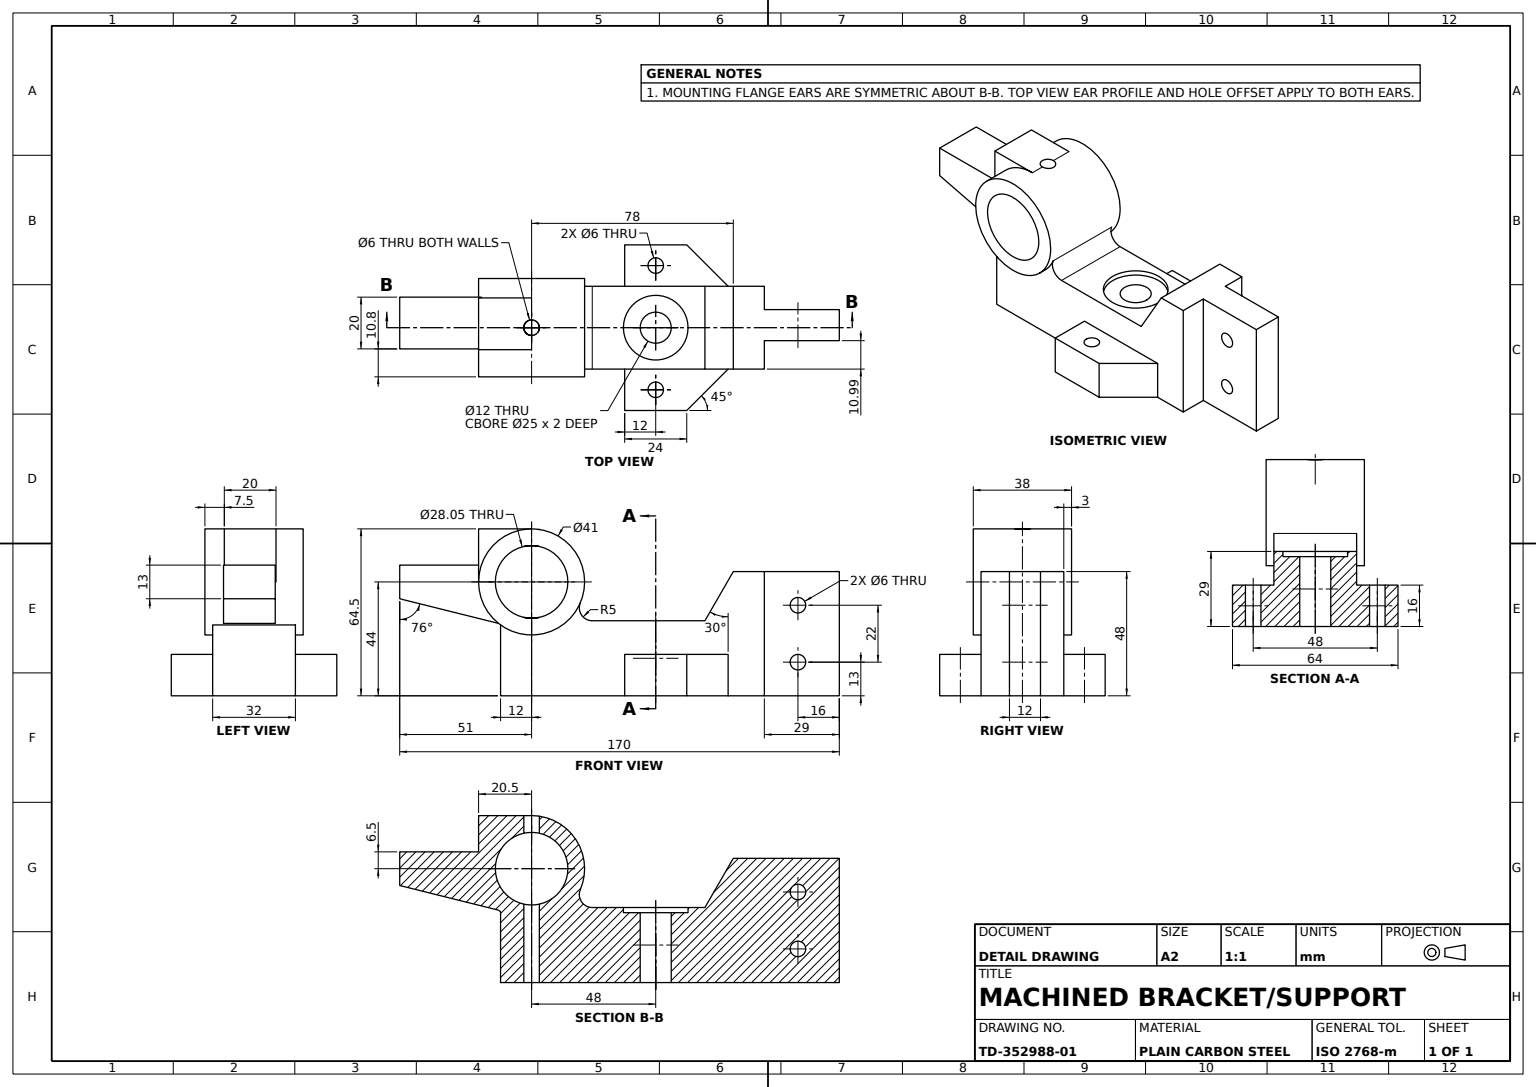
SolidWorks part; units mm, degrees
material "Plain Carbon Steel"
ref_plane "Front Plane" through (0, 0, 0) normal (0, 0, 1) x (1, 0, 0)
ref_plane "Top Plane" through (0, 0, 0) normal (0, 1, 0) x (1, 0, 0)
ref_plane "Right Plane" through (0, 0, 0) normal (1, 0, 0) x (0, 0, -1)
sketch "Base Block Sketch" plane through (0, 0, 0) normal (0, 1, 0) x (1, 0, 0)
  line L0 (-16.6126, 0) -> (35.5105, 0) construction
  line L1 (12, 0) -> (41, 0)
  line L3 (12, 12) -> (41, 12)
  line L4 (41, 0) -> (41, 12)
  line L9 (0, 23.3887) -> (0, -17.813) construction
  line L10 (0, 6) -> (46.308, 6) construction
  line L11 (0, -10.986) -> (12, -10.986)
  line L12 (0, -10.986) -> (0, 21.014)
  line L13 (0, 21.014) -> (12, 21.014)
  line L14 (12, -10.986) -> (12, 0)
  line L15 (12, 12) -> (12, 21.014)
  dimension "D1" = 12
  dimension "D2" = 41
  dimension "D3" = 12
  dimension "D4" = 32
  dimension "D5" = 10.986
  dimension "D6" = 2.3746
  dimension "D7" = 6.827
  dimension "D8" = 16.6126
  dimension "D9" = 5.4895
  dimension "D10" = 6
extrude "Base Block 48mm" add sketch "Base Block Sketch" along normal blind 48
sketch "Base Notch Sketch" plane through (0, 0, 0) normal (0, 0, 1) x (1, 0, 0)
  line L0 (25, 53.5167) -> (25, -6.2579) construction
  line L4 (12, 0) -> (41, 0) construction
  circle A0 centre (25, 35) radius 3
  circle A1 centre (25, 13) radius 3
  dimension "D4" = 6
  dimension "D1" = 25
  dimension "D2" = 22
  dimension "D3" = 13
extrude "Base Notch Cut" cut sketch "Base Notch Sketch" against normal through all
sketch "Angled Arm Sketch" plane through (0, 0, 10.986) normal (0, 0, 1) x (1, 0, 0)
  line L0 (0, 48) -> (-10.9697, 29)
  line L1 (-10.9697, 29) -> (-90, 29)
  line L2 (-90, 29) -> (-90, 0)
  line L3 (-90, 0) -> (0, 0)
  line L4 (12, 48) -> (12, 0) construction
  line L5 (0, 0) -> (0, 48)
  dimension "D1" = 90
  dimension "D2" = 30
  dimension "D3" = 29
extrude "Angled Arm 30deg" add sketch "Angled Arm Sketch" against normal blind 32
sketch "Mounting Flange Sketch" plane through (0, 0, 10.986) normal (0, 0, 1) x (1, 0, 0)
  line L0 (-78, 0) -> (-78, 44) construction
  line L1 (-90, 0) -> (12, 0) construction
  circle A0 centre (-78, 44) radius 20.5
  circle A1 centre (-78, 44) radius 14
  dimension "D3" = 41
  dimension "D4" = 28
  dimension "D1" = 12
  dimension "D2" = 44
extrude "Mounting Flange" add sketch "Mounting Flange Sketch" against normal blind 35 and the other way blind 3
sketch "Raised Block Sketch" plane through (0, 0, 0) normal (0, -1, 0) x (1, 0, 0)
  line L0 (-90, 10.986) -> (12, 10.986) construction
  line L2 (-18, 30.3579) -> (-18, -45.3477) construction
  line L3 (-2, 30.3579) -> (-2, -45.3477) construction
  line L4 (-42, -37.014) -> (-18, -37.014)
  line L8 (-42, -21.014) -> (-42, -37.014)
  line L9 (-18, -37.014) -> (-2, -21.014)
  line L10 (-2, -21.014) -> (-42, -21.014)
  line L11 (41, -6) -> (-93.5866, -6) construction
  line L12 (41, 0) -> (41, -12) construction
  line L16 (-42, 10.986) -> (-2, 10.986)
  line L18 (-2, 10.986) -> (-18, 26.986)
  line L19 (-18, 26.986) -> (-42, 26.986)
  line L20 (-42, 26.986) -> (-42, 10.986)
  dimension "D1" = 40
  dimension "D2" = 24
  dimension "D3" = 16
  dimension "D4" = 16
  dimension "D5" = 24
  dimension "D6" = 16
  dimension "D7" = 16
  dimension "D8" = 16
  dimension "D9" = 43
  dimension "D10" = 19.372
  dimension "D11" = 32
  dimension "D12" = 56.3337
  dimension "D13" = 134.5866
  dimension "D14" = 32
extrude "Raised Block 16mm" add sketch "Raised Block Sketch" against normal blind 16
sketch "Pocket Sketch" plane through (0, 29, 0) normal (0, 1, 0) x (1, 0, 0)
  line L0 (-30, 46.2556) -> (-30, -37.2312) construction
  line L3 (-42, -26.986) -> (-42, -10.986) construction
  line L4 (-18, -26.986) -> (-42, -26.986) construction
  line L5 (-42, 37.014) -> (-18, 37.014) construction
  line L6 (-57.5, 5.014) -> (-10.9697, 5.014) construction
  line L7 (-57.5, -13.986) -> (-57.5, 24.014) construction
  line L8 (-10.9697, 21.014) -> (-10.9697, -10.986) construction
  line L9 (-10.9697, 21.014) -> (-64.0268, 21.014) construction
  line L10 (-42, -10.986) -> (-2, -10.986) construction
  circle A0 centre (-30, -18.986) radius 3.1771
  circle A1 centre (-30, 29.014) radius 3.6319
  circle A2 centre (-30, 5.014) radius 12.5
  dimension "D7" = 25
  dimension "D8" = 6.3542
  dimension "D9" = 7.2639
  dimension "D1" = 12
  dimension "D2" = 48
  dimension "D3" = 8
  dimension "D4" = 8
  dimension "D5" = 16
  dimension "D6" = 16
extrude "Pocket Cut 2mm" cut sketch "Pocket Sketch" against normal blind 2
sketch "Slot Sketch" plane through (0, 27, 0) normal (0, 1, 0) x (1, 0, 0)
  line L0 (-42, 37.014) -> (-18, 37.014) construction
  line L1 (-18, -26.986) -> (-42, -26.986) construction
  circle A0 centre (-30, 5.014) radius 6
  circle A1 centre (-30, -18.986) radius 3
  circle A2 centre (-30, 29.014) radius 3
  dimension "D3" = 12
  dimension "D4" = 6
  dimension "D5" = 6
  dimension "D1" = 8
  dimension "D2" = 8
extrude "Slot Cut" cut sketch "Slot Sketch" against normal through all
sketch "Channel Sketch" plane through (0, 29, 0) normal (0, 1, 0) x (1, 0, 0)
  line L0 (-30, 5.014) -> (-30, 45.4469) construction
  line L1 (-30, 45.4469) -> (-78, 45.4469) construction
  line L2 (-78, 45.4469) -> (-78, -30.6069) construction
  line L3 (-98.5, 24.014) -> (-98.5, -13.986) construction
  line L5 (-10.9697, 21.014) -> (-64.0268, 21.014) construction
  circle A0 centre (-78, 5.014) radius 3
  dimension "D5" = 6
  dimension "D1" = 20.5
  dimension "D2" = 48
  dimension "D3" = 24.4328
extrude "Channel Cut" cut sketch "Channel Sketch" against normal through all both and the other way through all
sketch "Lug A Sketch" plane through (0, 0, 10.986) normal (0, 0, 1) x (1, 0, 0)
  line L0 (-78, 102.5038) -> (-78, -14.5038) construction
  line L1 (12, 48) -> (12, 0) construction
  line L3 (-90, 64.5) -> (-78, 64.5)
  line L4 (-90, 60.6208) -> (-90, 64.5)
  circle A0 centre (-78, 44) radius 14 construction
  circle A2 centre (-78, 44) radius 20.5 construction
  arc A4 (-78, 64.5) -> (-90, 60.6208) centre (-78, 44) ccw
  dimension "D1" = 102
extrude "Lug A" add sketch "Lug A Sketch" against normal blind 20 from offset 7.5 offset against normal yes
sketch "Lug B Sketch" plane through (0, 0, 10.986) normal (0, 0, 1) x (1, 0, 0)
  line L0 (-98.5, 44) -> (-98.5, 64.5)
  line L1 (-90, 64.5) -> (-98.5, 64.5)
  line L2 (-90, 64.5) -> (-90, 60.6208)
  line L4 (-2, 0) -> (12, 0) construction
  circle A0 centre (-78, 44) radius 20.5 construction
  arc A1 (-90, 60.6208) -> (-90, 27.3792) centre (-78, 44) ccw
  circle A2 centre (-78, 44) radius 20.5
  arc A3 (-90, 60.6208) -> (-98.5, 44) centre (-78, 44) ccw
  dimension "D1" = 0
  dimension "D2" = 60.6208
extrude "Lug B" add sketch "Lug B Sketch" against normal blind 20 from offset 7.5 contours A3 L0 L1 L2 offset against normal yes
sketch "Lug C Sketch" plane through (0, 0, 13.986) normal (0, 0, 1) x (1, 0, 0)
  line L0 (-78, 44) -> (-129, 44) construction
  line L1 (-129, 50.5) -> (-129, 37.5)
  line L2 (-129, 37.5) -> (-90, 27.7762)
  line L3 (-90, 27.3792) -> (-90, 0) construction
  line L5 (-90, 50.5) -> (-90, 27.7762)
  line L6 (-156.5568, 44) -> (-74.7731, 44) construction
  line L7 (-129, 50.5) -> (-90, 50.5)
  circle A0 centre (-78, 44) radius 20.5 construction
  dimension "D1" = 6.5
  dimension "D2" = 104
  dimension "D3" = 51
extrude "Lug C" add sketch "Lug C Sketch" against normal blind 20 from offset 10.8 offset against normal yes
sketch "Flange Hole Sketch" plane through (0, 0, 13.986) normal (0, 0, 1) x (1, 0, 0)
  circle A0 centre (-78, 44) radius 14.0251
  dimension "D1" = 28.0502
  dimension "D2" = 78
  dimension "D3" = 44
extrude "Flange Hole" cut sketch "Flange Hole Sketch" against normal through all both
sketch "Lug A Hole Sketch" plane through (0, 64.5, 0) normal (0, 1, 0) x (1, 0, 0)
  line L0 (-78, 8.014) -> (-78, 2.014) construction
  circle A0 centre (-78, 5.014) radius 3
  dimension "D1" = 6
extrude "Lug A Hole" cut sketch "Lug A Hole Sketch" against normal through all both
fillet "Arm Fillet R5" radius 5 1 edges at (-64.0268, 29, -5.014)
